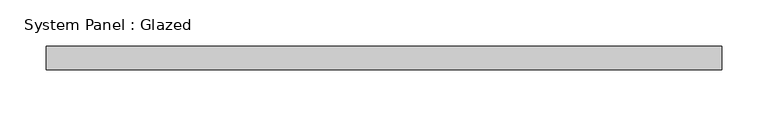
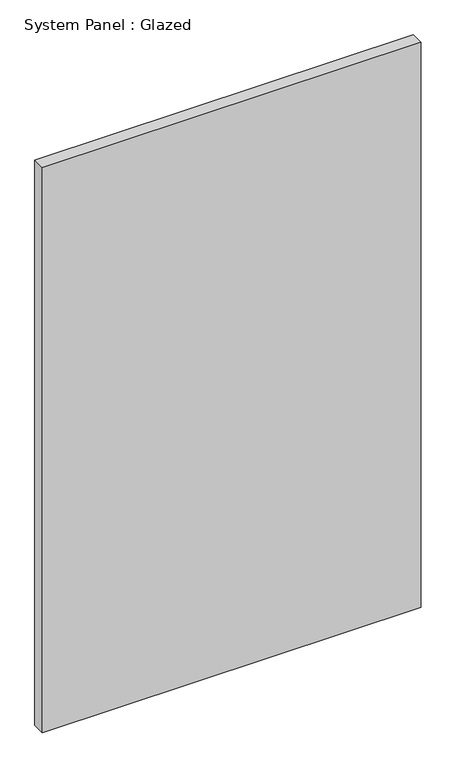
"""IFC4 building model written with IfcOpenShell, lengths in millimetres: plate geometry, System Panel : Glazed."""

from ifc_helpers import new_model, si_unit, origin, origin_with_axes, place, context, project, spatial, polyline, outline, extrude, source, transform, mapped, element, save


def system_panel_glazed_ccf5e832(model_context):
    return source(origin(), model_context, "Body", "SweptSolid", [
        extrude(outline(polyline([(366.1833333, 19.05), (-366.1833333, 19.05), (-366.1833333, 44.45), (366.1833333, 44.45), (366.1833333, 19.05)])), origin_with_axes(), (0.0, 0.0, 1.0), 1155.7),
    ])


if __name__ == "__main__":
    model = new_model("IFC4")
    model_context = context("Model", 3, world=origin())
    ifc_project = project(units=[si_unit("LENGTHUNIT", "METRE", prefix="MILLI")], contexts=[model_context])
    site = spatial("IfcSite", under=ifc_project)
    building = spatial("IfcBuilding", under=site)
    placement = place(None, origin())
    system_panel_glazed_shape = system_panel_glazed_ccf5e832(model_context)
    element("IfcPlate", 1, ObjectType="System Panel : Glazed", at=placement, inside=building, context=model_context, shape_type="MappedRepresentation", body=[
        mapped(system_panel_glazed_shape, transform((0.0, 0.0, 0.0), x_axis=(1.0, 0.0, 0.0), y_axis=(0.0, 1.0, 0.0), z_axis=(0.0, 0.0, 1.0))),
    ])
    save(model, "model.ifc")

# Revit data of these elements
# Type "System Panel : Glazed"
#   Construction Type Id = "GSP4R"
#   Analytic Construction = "1/8 in Pilkington single glazing"
#   Visual Light Transmittance = 0.9
#   Solar Heat Gain Coefficient = 0.86
#   Heat Transfer Coefficient (U) = 1.18115 BTU/(h·ft²·°F)
# Element 1 (IfcPlate, "System Panel : Glazed")
#   Materials on its faces: "Glass"
# Materials
#   "Glass": class "Glass", colour RGB 0 128 192, transparency 0.75, Description = "Soda Lime Glass", Cost = 0
